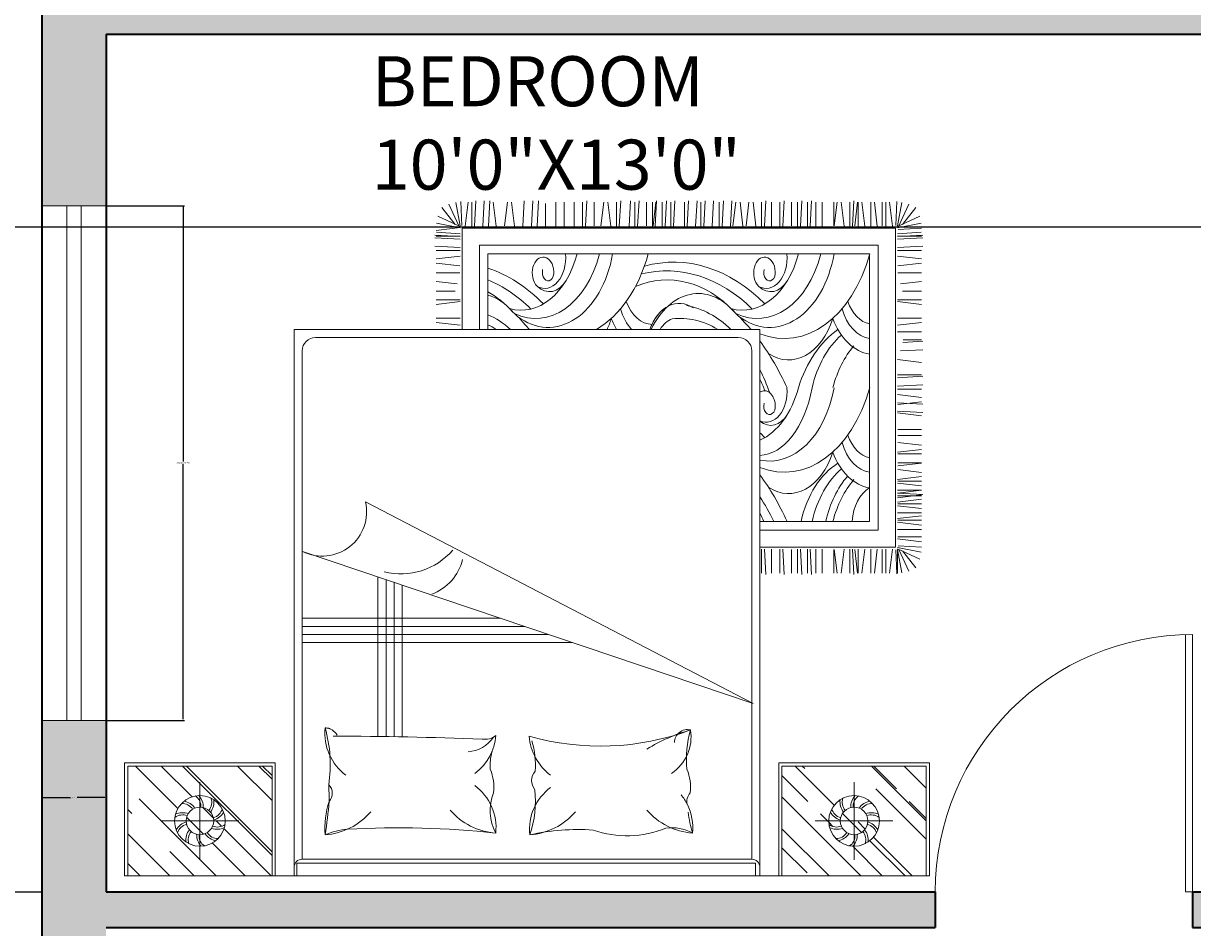
# Model space of a CAD drawing. Units: inches. Extents: x 2540 to 3167, y 3083 to 4007.
# Tile 5 of 15: x 2634 to 2798, y 3416 to 3542. Entities that reach past the tile are written whole.
import ezdxf

# ---------------------------------------------------------------- set-up
doc = ezdxf.new("R2010")
doc.units = ezdxf.units.IN
for name, color, linetype, lineweight in [('A-ANNO-DIMS', 2, 'Continuous', 18), ('A-AREA-IDEN', 7, 'Continuous', 18), ('A-DOOR', 4, 'Continuous', 18), ('A-FLOR-EDGE', 7, 'Continuous', 25), ('A-FURN', 8, 'Continuous', 13), ('A-GLAZ', 4, 'Continuous', 18)]:
    doc.layers.add(name, color=color, linetype=linetype, lineweight=lineweight)
doc.layers.add('A-WALL', color=143, linetype='Continuous', lineweight=35, true_color=0x7aafdf)
doc.layers.add('A-WALL-PATT', color=143, linetype='Continuous', lineweight=13, true_color=0x7aafdf)
doc.styles.get("Standard").update_dxf_attribs({"font": 'arial.ttf'})
doc.dimstyles.get("Standard").update_dxf_attribs({"dimtxt": 0.18, "dimasz": 0.18, "dimexe": 0.18, "dimexo": 0.0625, "dimgap": 0.09, "dimtad": 0, "dimtih": 1, "dimtoh": 1, "dimdec": 4, "dimzin": 0, "dimdsep": 46, "dimtxsty": 'Standard', "dimcen": 0.09, "dimadec": 0, "dimazin": 0, "dimtfac": 1, "dimtdec": 4, "dimtofl": 0, "dimtmove": 0, "dimatfit": 3, "dimfxl": 1, "dimtolj": 1, "dimtzin": 0, "dimarcsym": 0})

# ---------------------------------------------------------------- blocks, each defined once
blk = doc.blocks.new('A$C64B41DC1')
for p, q in [((0, 2.5079), (2.9903, 2.5079)), ((0, 2.0879), (0, 2.5079)), ((0.012, 2.4618), (0.0581, 2.5079)), ((0.012, 2.3515), (0.1684, 2.5079)), ((0.012, 2.0999), (0.012, 2.5079)), ((0.0543, 2.2213), (0.3409, 2.5079)), ((0.1689, 2.4179), (0.2589, 2.5079)), ((0.3265, 2.386), (0.4484, 2.5079)), ((0.3699, 2.3332), (0.5445, 2.5079)), ((0.548, 2.5079), (0.548, 2.0999)), ((0.56, 2.5079), (0.56, 2.0879)), ((0.6301, 2.5079), (0.6301, 0.4779)), ((0.6401, 2.461), (0.6401, 2.5079)), ((0.6401, 2.5079), (2.344, 2.5079)), ((2.344, 2.5079), (2.3601, 2.5079)), ((2.344, 2.5079), (2.344, 2.461)), ((2.3601, 2.5079), (2.3601, 2.4761)), ((2.3601, 0.4779), (2.3601, 2.5079)), ((2.4303, 2.5079), (2.4303, 2.0879)), ((2.4423, 2.5079), (2.4423, 2.0999)), ((2.4423, 2.3333), (2.6169, 2.5079)), ((2.4423, 2.2145), (2.7357, 2.5079)), ((2.4423, 2.404), (2.5354, 2.4971)), ((2.705, 2.398), (2.8149, 2.5079)), ((2.7691, 2.3772), (2.8998, 2.5079)), ((2.7819, 2.3646), (2.9252, 2.5079)), ((2.9783, 2.0999), (2.9783, 2.5079)), ((2.9903, 2.0879), (2.9903, 2.5079)), ((0.2157, 2.0999), (0.548, 2.4322)), ((0.2804, 2.1597), (0.2804, 2.4481)), ((2.344, 2.461), (0.6401, 2.461)), ((0.6601, 2.4461), (1.4951, 2.4461)), ((0.6601, 2.4461), (0.6601, 0.5579)), ((1.4951, 2.4461), (0.6697, 2.4461)), ((2.3301, 2.4461), (1.4951, 2.4461)), ((2.3301, 0.5579), (2.3301, 2.4461)), ((2.7099, 2.1597), (2.7099, 2.4481)), ((0.2299, 2.0999), (0.548, 2.418)), ((0.2311, 2.2906), (0.2937, 2.3532)), ((2.6674, 2.2756), (2.7382, 2.3464)), ((2.7914, 2.1846), (2.9783, 2.3715)), ((0.1362, 2.3039), (0.4246, 2.3039)), ((0.3405, 2.3039), (0.3605, 2.3238)), ((2.8541, 2.3039), (2.5657, 2.3039)), ((2.5849, 2.2779), (2.6158, 2.3088)), ((2.6158, 2.3088), (2.6313, 2.3243)), ((2.7249, 2.3076), (2.7512, 2.3339)), ((2.7746, 2.0999), (2.9783, 2.3036)), ((0.012, 2.261), (0.0275, 2.2765)), ((0.2905, 2.2539), (0.3304, 2.2938)), ((2.9144, 2.2312), (2.9783, 2.2951)), ((0.0404, 2.0999), (0.1982, 2.2578)), ((0.4194, 2.0999), (0.548, 2.2285)), ((2.4423, 2.1353), (2.5382, 2.2312)), ((2.4918, 2.0999), (2.6366, 2.2447)), ((0.1365, 2.0999), (0.251, 2.2144)), ((2.7831, 2.0999), (2.8678, 2.1846)), ((2.8962, 2.0999), (2.9783, 2.182)), ((0.4986, 2.0999), (0.548, 2.1493)), ((0.5127, 2.0999), (0.548, 2.1352)), ((0.56, 2.0879), (0, 2.0879)), ((0.548, 2.0999), (0.012, 2.0999)), ((2.4303, 2.0879), (2.9903, 2.0879)), ((2.4423, 2.0999), (2.9783, 2.0999)), ((2.5172, 2.0999), (2.5269, 2.1096)), ((0.9415, 1.9902), (0.9415, 1.3975)), ((0.9715, 1.9906), (0.9715, 1.4076)), ((1.0015, 1.991), (1.0015, 1.4177)), ((1.0315, 1.9916), (1.0315, 1.4279)), ((2.3349, 1.8678), (0.6613, 1.3029)), ((0.8956, 1.1191), (2.3349, 1.8678)), ((1.6636, 1.6412), (0.6601, 1.6412)), ((1.5748, 1.6112), (0.6601, 1.6112)), ((2.3665, 1.295), (2.3665, 1.3839)), ((2.377, 1.295), (2.3822, 1.3891)), ((2.4032, 1.295), (2.4032, 1.3839)), ((2.4346, 1.295), (2.4346, 1.3839)), ((2.4451, 1.295), (2.4503, 1.3891)), ((2.4774, 1.2957), (2.4774, 1.3837)), ((2.5, 1.295), (2.5, 1.3839)), ((2.5105, 1.295), (2.5157, 1.3891)), ((2.5367, 1.295), (2.5367, 1.3839)), ((2.5471, 1.295), (2.5524, 1.3891)), ((2.5681, 1.295), (2.5681, 1.3839)), ((2.5918, 1.295), (2.5918, 1.3839)), ((2.6346, 1.2957), (2.6346, 1.3837)), ((2.6362, 1.2957), (2.6467, 1.3839)), ((2.6729, 1.295), (2.6624, 1.3839)), ((2.6938, 1.295), (2.6938, 1.3839)), ((2.7043, 1.295), (2.7095, 1.3891)), ((2.7127, 1.2957), (2.7232, 1.3839)), ((2.7253, 1.295), (2.7253, 1.3839)), ((2.7494, 1.295), (2.7389, 1.3839)), ((2.7718, 1.295), (2.7718, 1.3839)), ((2.7959, 1.295), (2.7854, 1.3839)), ((2.8146, 1.2957), (2.8146, 1.3837)), ((2.8146, 1.2957), (2.8146, 1.3837)), ((2.8282, 1.295), (2.8282, 1.3839)), ((2.8282, 1.295), (2.8282, 1.3839)), ((2.8523, 1.295), (2.8418, 1.3839)), ((2.8523, 1.295), (2.8418, 1.3839)), ((2.8653, 1.2966), (2.8688, 1.3861)), ((2.8711, 1.2957), (2.8711, 1.3837)), ((2.8711, 1.2957), (2.8875, 1.3822)), ((2.8765, 1.2958), (2.9132, 1.3758)), ((2.8893, 1.3011), (2.9394, 1.3636)), ((2.8713, 1.2927), (2.954, 1.3315)), ((2.8717, 1.2884), (2.9588, 1.3058)), ((2.3601, 1.2873), (2.8639, 1.2873)), ((2.8639, 1.2873), (2.8639, 0.1018)), ((2.8716, 1.2565), (2.9605, 1.2669)), ((2.8744, 1.2817), (2.9603, 1.2869)), ((2.3601, 1.2233), (2.7999, 1.2233)), ((2.7999, 1.2233), (2.7999, 0.1658)), ((2.8716, 1.2212), (2.9605, 1.2212)), ((2.8723, 1.2489), (2.9603, 1.2489)), ((2.3601, 1.1913), (2.7679, 1.1912)), ((2.7679, 1.1912), (2.7679, 0.1978)), ((2.8716, 1.1947), (2.9605, 1.2052)), ((2.8716, 1.181), (2.9605, 1.1705)), ((2.8723, 1.1872), (2.9603, 1.1872)), ((2.8716, 1.1595), (2.9605, 1.1595)), ((2.8716, 1.133), (2.9605, 1.1435)), ((2.8716, 1.1193), (2.9605, 1.1088)), ((2.8716, 1.1035), (2.9605, 1.093)), ((2.8716, 1.0965), (2.9605, 1.0965)), ((2.8716, 1.086), (2.9657, 1.0913)), ((2.8723, 1.1255), (2.9603, 1.1255)), ((2.8723, 1.0858), (2.9605, 1.0753)), ((2.8716, 1.0756), (2.9605, 1.0756)), ((2.8716, 1.0491), (2.9605, 1.0596)), ((2.8716, 1.0354), (2.9605, 1.0249)), ((2.8723, 1.0416), (2.9603, 1.0416)), ((2.8723, 0.9987), (2.9605, 1.0092)), ((2.8723, 0.985), (2.9605, 0.9745)), ((2.8723, 0.9735), (2.9603, 0.9735)), ((2.8716, 0.9346), (2.9605, 0.9241)), ((2.8723, 0.9408), (2.9603, 0.9408)), ((2.8723, 0.8979), (2.9605, 0.9084)), ((2.8723, 0.8726), (2.9603, 0.8726)), ((2.8723, 0.8505), (2.9603, 0.8505)), ((2.8716, 0.7885), (2.9605, 0.799)), ((2.8716, 0.7818), (2.9657, 0.787)), ((2.8716, 0.7503), (2.9657, 0.7556)), ((2.8723, 0.7571), (2.9605, 0.7466)), ((2.8716, 0.7204), (2.9605, 0.7309)), ((2.8716, 0.6995), (2.9605, 0.6995)), ((2.8716, 0.689), (2.9657, 0.6838)), ((2.8716, 0.6576), (2.9657, 0.6523)), ((2.8716, 0.6471), (2.9605, 0.6471)), ((2.8716, 0.5903), (2.9605, 0.6007)), ((2.882, 0.5582), (2.9657, 0.5536)), ((2.8909, 0.5263), (2.9657, 0.5222)), ((0.6301, 0.4779), (2.3601, 0.4779)), ((0.7101, 0.5079), (2.2801, 0.5079)), ((1.2542, 0.1018), (1.2542, 0.4779)), ((1.3182, 0.1658), (1.3182, 0.4779)), ((1.3502, 0.1978), (1.3502, 0.4779)), ((2.8716, 0.4877), (2.9603, 0.4877)), ((2.8928, 0.5169), (2.9605, 0.5169)), ((1.2465, 0.4625), (1.1576, 0.452)), ((1.2465, 0.4365), (1.1577, 0.4365)), ((2.8716, 0.4625), (2.9605, 0.452)), ((2.8716, 0.4365), (2.9603, 0.4365)), ((1.2465, 0.3746), (1.1576, 0.3851)), ((1.2465, 0.3684), (1.1577, 0.3684)), ((2.8716, 0.3746), (2.9605, 0.3851)), ((2.8716, 0.3684), (2.9603, 0.3684)), ((1.2355, 0.3092), (1.1576, 0.3)), ((1.2285, 0.3357), (1.1577, 0.3357)), ((2.8826, 0.3092), (2.9605, 0.3)), ((2.8896, 0.3357), (2.9603, 0.3357)), ((1.2457, 0.2676), (1.1577, 0.2676)), ((2.8723, 0.2676), (2.9603, 0.2676)), ((1.2457, 0.2423), (1.1576, 0.2319)), ((2.8723, 0.2423), (2.9605, 0.2319)), ((1.2465, 0.1742), (1.1524, 0.169)), ((1.2465, 0.2057), (1.1576, 0.2161)), ((1.2465, 0.1847), (1.1576, 0.1847)), ((2.7679, 0.1978), (1.3502, 0.1978)), ((2.8716, 0.2057), (2.9605, 0.2161)), ((2.8716, 0.1847), (2.9605, 0.1847)), ((2.8716, 0.1742), (2.9657, 0.169)), ((1.2465, 0.1428), (1.1524, 0.1376)), ((1.2465, 0.1334), (1.1524, 0.1281)), ((1.2465, 0.1323), (1.1576, 0.1323)), ((1.2465, 0.1323), (1.1576, 0.1323)), ((2.7999, 0.1658), (1.3182, 0.1658)), ((2.8716, 0.1428), (2.9657, 0.1376)), ((2.8716, 0.1334), (2.9657, 0.1281)), ((2.8716, 0.1323), (2.9605, 0.1323)), ((1.2465, 0.1), (1.1576, 0.1105)), ((1.2465, 0.1229), (1.1588, 0.1168)), ((1.2464, 0.1007), (1.1592, 0.0833)), ((1.2468, 0.0964), (1.1641, 0.0576)), ((1.2288, 0.088), (1.1787, 0.0255)), ((1.2415, 0.0933), (1.2049, 0.0133)), ((1.247, 0.0934), (1.2306, 0.0069)), ((1.2527, 0.0925), (1.2493, 0.003)), ((2.8639, 0.1018), (1.2542, 0.1018)), ((1.2658, 0.0941), (1.2762, 0.0052)), ((1.2899, 0.0941), (1.2899, 0.0052)), ((1.2999, 0.0941), (1.3051, 0)), ((1.3313, 0.0941), (1.3365, 0)), ((1.3523, 0.0941), (1.3575, 0)), ((1.3804, 0.0941), (1.3699, 0.0052)), ((1.4119, 0.0934), (1.4223, 0.0052)), ((1.4485, 0.0941), (1.438, 0.0052)), ((1.48, 0.0941), (1.4852, 0)), ((1.5114, 0.0941), (1.5166, 0)), ((1.5323, 0.0941), (1.5376, 0)), ((1.5638, 0.0941), (1.5638, 0.0105)), ((1.6021, 0.0941), (1.6021, 0.0052)), ((1.6336, 0.0941), (1.6336, 0.0052)), ((1.6702, 0.0941), (1.6702, 0.0052)), ((1.7017, 0.0941), (1.7017, 0.0052)), ((1.7122, 0.0941), (1.7174, 0)), ((1.7445, 0.0934), (1.7445, 0.0054)), ((1.7698, 0.0934), (1.7803, 0.0052)), ((1.8065, 0.0941), (1.796, 0.0052)), ((1.8274, 0.0941), (1.8274, 0.0052)), ((1.8379, 0.0941), (1.8431, 0)), ((1.8746, 0.0941), (1.8798, 0)), ((1.8955, 0.0941), (1.8955, 0.0052)), ((1.906, 0.0941), (1.9113, 0)), ((1.9384, 0.0934), (1.9384, 0.0054)), ((1.9609, 0.0941), (1.9609, 0.0052)), ((1.9636, 0.0934), (1.9741, 0.0052)), ((1.9714, 0.0941), (1.9766, 0)), ((1.9976, 0.0941), (1.9976, 0.0052)), ((2.0081, 0.0941), (2.0133, 0)), ((2.029, 0.0941), (2.029, 0.0052)), ((2.0395, 0.0941), (2.0447, 0)), ((2.0797, 0.0941), (2.0797, 0.0052)), ((2.0902, 0.0941), (2.0954, 0)), ((2.1216, 0.0941), (2.1269, 0)), ((2.1412, 0.0941), (2.1412, 0.0052)), ((2.1517, 0.0941), (2.1569, 0)), ((2.1831, 0.0941), (2.1884, 0)), ((2.2093, 0.0941), (2.2093, 0.0052)), ((2.2198, 0.0941), (2.225, 0)), ((2.2512, 0.0941), (2.2565, 0)), ((2.2603, 0.0934), (2.2707, 0.0052)), ((2.2969, 0.0941), (2.2864, 0.0052)), ((2.3089, 0.0934), (2.3193, 0.0052)), ((2.3455, 0.0941), (2.3351, 0.0052)), ((2.3665, 0.0941), (2.3665, 0.0052)), ((2.377, 0.0941), (2.3822, 0)), ((2.4032, 0.0941), (2.4032, 0.0052)), ((2.4346, 0.0941), (2.4346, 0.0052)), ((2.4451, 0.0941), (2.4503, 0)), ((2.4774, 0.0934), (2.4774, 0.0054)), ((2.5, 0.0941), (2.5, 0.0052)), ((2.5105, 0.0941), (2.5157, 0)), ((2.5367, 0.0941), (2.5367, 0.0052)), ((2.5471, 0.0941), (2.5524, 0)), ((2.5681, 0.0941), (2.5681, 0.0052)), ((2.5918, 0.0941), (2.5918, 0.0052)), ((2.6346, 0.0934), (2.6346, 0.0054)), ((2.6362, 0.0934), (2.6467, 0.0052)), ((2.6729, 0.0941), (2.6624, 0.0052)), ((2.6938, 0.0941), (2.6938, 0.0052)), ((2.7043, 0.0941), (2.7095, 0)), ((2.7127, 0.0934), (2.7232, 0.0052)), ((2.7253, 0.0941), (2.7253, 0.0052)), ((2.7494, 0.0941), (2.7389, 0.0052)), ((2.7718, 0.0941), (2.7718, 0.0052)), ((2.7959, 0.0941), (2.7854, 0.0052)), ((2.8146, 0.0934), (2.8146, 0.0054)), ((2.8282, 0.0941), (2.8282, 0.0052)), ((2.8523, 0.0941), (2.8418, 0.0052)), ((2.8653, 0.0925), (2.8688, 0.003)), ((2.8711, 0.0934), (2.8875, 0.0069)), ((2.8713, 0.0964), (2.954, 0.0576)), ((2.8716, 0.1229), (2.9593, 0.1168)), ((2.8717, 0.1007), (2.9588, 0.0833)), ((2.8744, 0.1074), (2.9603, 0.1022)), ((2.8765, 0.0933), (2.9132, 0.0133)), ((2.8893, 0.088), (2.9394, 0.0255))]:
    blk.add_line(p, q)
at = {"ltscale": 10}
for p, q in [((1.4859, 1.5812), (0.6601, 1.5812)), ((1.397, 1.5512), (0.6601, 1.5512))]:
    blk.add_line(p, q, dxfattribs=at)
for centre, radius in [((0.2804, 2.3039), 0.0942), ((2.7099, 2.3039), 0.0942), ((0.2804, 2.3039), 0.051), ((2.7099, 2.3039), 0.051)]:
    blk.add_circle(centre, radius)
for centre, radius, start, end in [((0.6601, 2.4761), 0.03, 180, 270), ((2.3301, 2.4761), 0.03, 270, 0), ((0.2828, 2.3731), 0.0462, 160.3002, 220.538), ((0.3286, 2.3561), 0.0605, 136.17, 182.4897), ((0.3231, 2.3585), 0.0462, 124.3002, 184.538), ((2.6672, 2.3585), 0.0462, 355.462, 55.6998), ((2.6617, 2.3561), 0.0605, 357.5103, 43.83), ((2.7075, 2.3731), 0.0462, 319.462, 19.6998), ((0.2417, 2.3614), 0.0462, 196.3002, 256.538), ((0.2887, 2.3745), 0.0605, 172.17, 218.4897), ((0.3501, 2.3178), 0.0605, 100.17, 146.4897), ((0.347, 2.323), 0.0462, 88.3002, 148.538), ((1.0526, 2.3302), 0.3085, 175.3048, 198.6942), ((-0.8702, 2.0941), 1.6364, 4.8098, 9.1892), ((0.8579, 2.6278), 0.2948, 247.5179, 264.267), ((0.728, 2.111), 0.245, 40.4189, 85.9871), ((1.0164, 5.7096), 3.3803, 266.8134, 276.1602), ((1.3963, 2.1044), 0.245, 94.0129, 139.5811), ((1.1858, 2.3288), 0.1943, 306.5711, 5.89), ((1.5348, 2.2652), 0.1767, 151.7736, 201.6983), ((1.6986, 2.3355), 0.1943, 174.11, 233.4289), ((1.1481, 2.2311), 0.3783, 353.4947, 19.1867), ((1.6871, 3.192), 0.8561, 257.7438, 273.6284), ((1.4882, 2.111), 0.245, 40.4189, 85.9871), ((1.8674, 1.9709), 0.3878, 68.2026, 108.9817), ((2.1269, 2.1044), 0.245, 94.0129, 139.5811), ((2.0342, 2.4856), 0.1563, 261.5958, 298.9092), ((1.9165, 2.3288), 0.1943, 333.7371, 5.89), ((2.6058, 2.2028), 0.517, 163.6046, 172.3273), ((2.6433, 2.323), 0.0462, 31.462, 91.6998), ((2.6402, 2.3178), 0.0605, 33.5103, 79.83), ((2.7016, 2.3745), 0.0605, 321.5103, 7.83), ((2.7486, 2.3614), 0.0462, 283.462, 343.6998), ((0.2457, 2.3659), 0.0605, 208.17, 254.4897), ((0.3449, 2.2742), 0.0605, 64.17, 110.4897), ((0.3455, 2.2802), 0.0462, 52.3002, 112.538), ((2.6448, 2.2802), 0.0462, 67.462, 127.6998), ((2.6454, 2.2742), 0.0605, 69.5103, 115.83), ((2.7446, 2.3659), 0.0605, 285.5103, 331.83), ((0.2153, 2.3276), 0.0462, 232.3002, 292.538), ((0.2158, 2.3336), 0.0605, 244.17, 290.4897), ((0.2138, 2.2848), 0.0462, 268.3002, 328.538), ((0.2779, 2.2347), 0.0462, 340.3002, 40.538), ((0.272, 2.2333), 0.0605, 352.17, 38.4897), ((0.3191, 2.2464), 0.0462, 16.3002, 76.538), ((0.3151, 2.2419), 0.0605, 28.17, 74.4897), ((2.6752, 2.2419), 0.0605, 105.5103, 151.83), ((2.6712, 2.2464), 0.0462, 103.462, 163.6998), ((2.7182, 2.2333), 0.0605, 141.5103, 187.83), ((2.7123, 2.2347), 0.0462, 139.462, 199.6998), ((2.7765, 2.2848), 0.0462, 211.462, 271.6998), ((2.7744, 2.3336), 0.0605, 249.5103, 295.83), ((2.775, 2.3276), 0.0462, 247.462, 307.6998), ((0.2107, 2.29), 0.0605, 280.17, 326.4897), ((0.2377, 2.2493), 0.0462, 304.3002, 4.538), ((0.2322, 2.2517), 0.0605, 316.17, 2.4897), ((0.7274, 2.2013), 0.0446, 314.4736, 42.1713), ((-1.6008, 2.277), 2.3618, 357.3905, 358.8876), ((1.9165, 2.3288), 0.1943, 320.9404, 333.7371), ((2.1347, 2.2313), 0.0459, 165.3506, 223.2684), ((2.7581, 2.2517), 0.0605, 177.5103, 223.83), ((2.7526, 2.2493), 0.0462, 175.462, 235.6998), ((2.7796, 2.29), 0.0605, 213.5103, 259.83), ((1.204, 2.1778), 0.1681, 337.017, 7.5368), ((1.5671, 2.1546), 0.0547, 142.0833, 220.902), ((1.9346, 2.1778), 0.1681, 337.017, 7.5368), ((0.9385, 1.978), 0.1943, 126.5711, 185.89), ((0.2688, 2.0945), 0.4956, 344.0243, 8.7071), ((1.7059, 1.9714), 0.204, 127.1197, 175.09), ((1.1858, 1.9714), 0.1943, 4.3181, 53.4289), ((1.5415, 2.0969), 0.1834, 175.2233, 196.23), ((1.1965, 2.0983), 0.3299, 343.7954, 3.5554), ((1.9394, 1.991), 0.1651, 351.2621, 55.7572), ((2.4617, 2.0719), 0.3745, 173.8296, 196.4356), ((1.2687, 1.9248), 0.1223, 33.628, 86.4744), ((0.7246, 18.8439), 16.8552, 270.17399, 272.05214), ((1.3401, 1.9404), 0.0603, 49.0991, 101.3702), ((1.7676, 1.0629), 0.9631, 69.6507, 105.9631), ((2.2748, 2.5795), 0.6373, 238.3499, 254.3137), ((2.0911, 2.0123), 0.0478, 179.7727, 283.8018), ((0.7417, 2.0149), 0.057, 273.4709, 328.5412), ((0.728, 2.2025), 0.245, 274.0129, 278.3417), ((1.0747, 1.2871), 0.1871, 14.1863, 69.1212), ((1.0274, 1.1334), 0.2527, 40.629, 104.3712), ((0.7347, 1.1553), 0.1649, 347.3109, 116.4454), ((0.7101, 0.5579), 0.05, 180, 270), ((2.2801, 0.5579), 0.05, 270, 0)]:
    blk.add_arc(centre, radius, start, end)
for centre, major_axis, ratio, start_param, end_param in [((1.9938, 1.6262), (0, -0.7531), 0.68, 0.797284, 0.954936), ((2.0643, 1.466), (0, -0.5322), 0.68, 7.239912, 7.311536), ((1.9052, 1.7397), (0, -0.9842), 0.68, 0.74745, 0.979724), ((2.7455, 1.3081), (0, 0.3614), 0.68, 1.900046, 2.742661), ((2.7868, 1.3081), (0, 0.3614), 0.68, 1.900046, 2.614747), ((2.8372, 1.3081), (0, 0.3614), 0.68, 1.900046, 2.479658), ((2.8607, 1.3211), (0, 0.3614), 0.68, 1.938265, 2.479658), ((2.8057, 1.2079), (0, -0.1524), 0.68, 4.821745, 5.895886), ((2.4665, 0.8216), (0, -0.2664), 0.68, 2.006169, 3.565187), ((2.4513, 0.5069), (0, 0.502), 0.68, 5.095327, 6.553458), ((2.7862, 0.8069), (0, -0.2615), 0.68, 3.244645, 4.205018), ((2.7784, 0.8289), (0, -0.1802), 0.68, 3.227058, 4.318474), ((2.396, 0.6032), (0, 0.3641), 0.68, -1.3172, 0.145284), ((2.3507, 0.5642), (0.0073, 0.3819), 0.56205, -1.21172, -0.009991), ((2.7821, 0.7971), (0, -0.1589), 0.68, 3.272942, 4.229533), ((2.2964, 0.5771), (0, -0.3263), 0.68, 1.938944, 2.850232), ((2.0403, 1.6015), (0, -0.8763), 0.68, 6.849801, 6.887077), ((2.4005, 0.7132), (0, -0.1214), 0.68, 2.284368, 3.652258), ((2.3834, 0.7081), (0, 0.1147), 0.68, 4.593909, 6.585576), ((2.3961, 0.7628), (0, -0.0317), 0.68, 1.462497, 5.046281), ((2.3774, 0.7653), (0, -0.0593), 0.68, 5.841311, 7.755362), ((1.9938, 1.1295), (-0.0678, 0.7439), 0.610498, 3.917146, 4.063997), ((2.0643, 0.9693), (0, -0.5322), 0.68, 7.239912, 7.336618), ((1.9052, 1.243), (0, -0.9842), 0.68, 0.74745, 0.979724), ((2.7455, 0.8114), (-0.0599, 0.3735), 0.695517, 1.775813, 2.548612), ((2.7868, 0.8114), (0, 0.3614), 0.68, 1.900046, 2.614747), ((2.8607, 0.8243), (0, 0.3614), 0.68, 1.938265, 2.479658), ((2.4665, 0.3249), (0, -0.2664), 0.68, 2.006169, 3.565187), ((2.7862, 0.3102), (0, -0.2615), 0.68, 3.244645, 4.205018), ((2.4513, 0.0102), (0, 0.502), 0.68, 5.095327, 6.553458), ((1.242, 0.9693), (0, -0.5322), 0.68, 6.586764, 6.677612), ((1.1714, 1.1295), (-0.1157, 0.7241), 0.59432, 3.291697, 3.50733), ((1.0828, 1.243), (0, -0.9842), 0.68, 0.565948, 0.680366), ((1.5283, 0.0674), (0, -0.3703), 0.68, 1.930561, 3.464283), ((1.5736, 0.1065), (0, 0.3641), 0.68, -1.3172, 0.476403), ((1.6289, 0.0102), (0, 0.502), 0.68, 6.655152, 6.661293), ((1.6289, 0.0102), (0, 0.502), 0.68, 5.095327, 5.911219), ((1.6442, 0.3249), (0, -0.2664), 0.68, 2.006169, 2.182797), ((1.9638, 0.3102), (0, -0.2615), 0.68, 4.015924, 4.205018), ((1.956, 0.3322), (0, -0.1802), 0.68, 3.770744, 4.318474), ((2.0606, 0.5616), (0, -0.1803), 0.68, 5.194792, 5.929328), ((2.0606, 0.5616), (0, -0.1803), 0.68, 5.194792, 6.723255), ((2.1315, 0.6603), (0, -0.3155), 0.68, 5.328638, 6.949396), ((2.0549, 0.5656), (0, -0.1303), 0.68, 5.450951, 6.054641), ((2.0643, 0.9693), (0, -0.5322), 0.68, 6.20013, 6.677612), ((1.9938, 1.1295), (-0.0678, 0.7439), 0.610498, 3.199135, 3.592282), ((1.9052, 1.243), (0, -0.9842), 0.68, 0.565948, 0.680366), ((2.3507, 0.0674), (0, -0.3703), 0.68, 1.930561, 3.464283), ((2.396, 0.1065), (0, 0.3641), 0.68, -1.3172, 0.476403), ((2.4513, 0.0102), (0, 0.502), 0.68, 6.655152, 6.661293), ((2.7784, 0.3322), (0, -0.1802), 0.68, 3.227058, 4.318474), ((1.9597, 0.3004), (0, -0.1589), 0.68, 3.14258, 4.229533), ((2.7821, 0.3004), (0, -0.1589), 0.68, 3.272942, 4.229533), ((1.1933, 0.9181), (0, -0.624), 0.68, 0.378672, 0.625379), ((1.3091, 0.6603), (0, -0.3155), 0.68, 6.475719, 6.949396), ((1.1911, 1.1066), (0, 0.8458), 0.68, 3.421828, 3.728616), ((1.474, 0.0804), (0, -0.3263), 0.68, 1.938944, 3.339184), ((2.0157, 0.9181), (0, -0.624), 0.68, -0.280078, 0.625379), ((2.0135, 1.1066), (0, 0.8458), 0.68, 2.978727, 3.728616), ((2.2964, 0.0804), (0, -0.3263), 0.68, 1.938944, 3.339184), ((1.2179, 1.1047), (0, -0.8763), 0.68, 6.507006, 6.887077), ((1.5781, 0.2165), (0, -0.1214), 0.68, 2.284368, 3.726131), ((2.0403, 1.1047), (0, -0.8763), 0.68, 6.099302, 6.887077), ((2.4005, 0.2165), (0, -0.1214), 0.68, 2.284368, 3.726131), ((1.555, 0.2685), (0, -0.0593), 0.68, 3.732151, 7.755362), ((1.561, 0.2114), (0, 0.1147), 0.68, 4.593909, 6.647252), ((2.3774, 0.2685), (0, -0.0593), 0.68, 3.732151, 7.755362), ((2.3834, 0.2114), (0, 0.1147), 0.68, 4.593909, 6.647252), ((1.5737, 0.2661), (0, -0.0317), 0.68, 1.462497, 5.046281), ((2.3961, 0.2661), (0, -0.0317), 0.68, 1.462497, 5.046281)]:
    blk.add_ellipse(centre, major_axis=major_axis, ratio=ratio, start_param=start_param, end_param=end_param)
blk = doc.blocks.new('DOOR-SWING-36IN')
for p, q in [((36, 0), (0, 0)), ((36, 1), (0.01, 1)), ((36, 1), (36, 0))]:
    blk.add_line(p, q)
blk.add_arc((36, 0), 36, 90, 180)
blk = doc.blocks.new('WIN-72IN')
for p, q in [((9, 72), (0, 72)), ((3.5, 0), (3.5, 72)), ((5.5, 0), (5.5, 72)), ((9, 0), (0, 0))]:
    blk.add_line(p, q)
blk = doc.blocks.new('*D27')
at = {"layer": 'A-ANNO-DIMS', "color": 0, "lineweight": -2, "transparency": 16777216}
for p, q in [((2645.57, 3516.71), (2656.49, 3516.71)), ((2656.31, 3516.53), (2656.31, 3480.9)), ((2656.31, 3444.89), (2656.31, 3480.53)), ((2645.57, 3444.71), (2656.49, 3444.71))]:
    blk.add_line(p, q, dxfattribs=at)
at = {"layer": 'A-ANNO-DIMS', "color": 0, "transparency": 16777216}
for points in [[(2656.28, 3516.53), (2656.34, 3516.53), (2656.31, 3516.71)], [(2656.28, 3444.89), (2656.34, 3444.89), (2656.31, 3444.71)]]:
    blk.add_solid(points, dxfattribs=at)
at = {"layer": 'Defpoints', "color": 0, "transparency": 16777216}
for p in [(2645.51, 3516.71), (2656.31, 3516.71), (2645.51, 3444.71)]:
    blk.add_point(p, dxfattribs=at)
at = {"layer": 'A-ANNO-DIMS', "color": 0, "transparency": 16777216, "insert": (2656.31, 3480.71), "char_height": 0.18, "attachment_point": 5}
blk.add_mtext('\\A1;WINDOW 72 TYP.', dxfattribs=at)
blk = doc.blocks.new('*D28')
at = {"layer": 'A-ANNO-DIMS', "color": 0, "lineweight": -2, "transparency": 16777216}
for p, q in [((2636.51, 3444.65), (2636.51, 3433.73)), ((2645.51, 3444.65), (2645.51, 3433.73)), ((2636.69, 3433.91), (2640.55, 3433.91)), ((2645.33, 3433.91), (2641.47, 3433.91))]:
    blk.add_line(p, q, dxfattribs=at)
at = {"layer": 'A-ANNO-DIMS', "color": 0, "transparency": 16777216}
for points in [[(2636.69, 3433.94), (2636.69, 3433.88), (2636.51, 3433.91)], [(2645.33, 3433.94), (2645.33, 3433.88), (2645.51, 3433.91)]]:
    blk.add_solid(points, dxfattribs=at)
at = {"layer": 'Defpoints', "color": 0, "transparency": 16777216}
for p in [(2636.51, 3444.71), (2645.51, 3444.71), (2645.51, 3433.91)]:
    blk.add_point(p, dxfattribs=at)
at = {"layer": 'A-ANNO-DIMS', "color": 0, "transparency": 16777216, "insert": (2641.01, 3433.91), "char_height": 0.18, "attachment_point": 5}
blk.add_mtext('\\A1;9 TYP.', dxfattribs=at)
blk = doc.blocks.new('*D44')
at = {"layer": 'A-ANNO-DIMS', "color": 0, "lineweight": -2, "transparency": 16777216}
for p, q in [((2771.45, 3964.71), (2540.23, 3964.71)), ((2540.41, 3964.53), (2540.41, 3545.4)), ((2540.41, 3125.89), (2540.41, 3545.03)), ((2810.45, 3125.71), (2540.23, 3125.71))]:
    blk.add_line(p, q, dxfattribs=at)
at = {"layer": 'A-ANNO-DIMS', "color": 0, "transparency": 16777216}
for points in [[(2540.38, 3964.53), (2540.44, 3964.53), (2540.41, 3964.71)], [(2540.38, 3125.89), (2540.44, 3125.89), (2540.41, 3125.71)]]:
    blk.add_solid(points, dxfattribs=at)
at = {"layer": 'Defpoints', "color": 0, "transparency": 16777216}
for p in [(2540.41, 3964.71), (2771.51, 3964.71), (2810.51, 3125.71)]:
    blk.add_point(p, dxfattribs=at)
at = {"layer": 'A-ANNO-DIMS', "color": 0, "transparency": 16777216, "insert": (2540.41, 3545.21), "char_height": 0.18, "attachment_point": 5}
blk.add_mtext('\\A1;839', dxfattribs=at)
blk = doc.blocks.new('*D57')
at = {"layer": 'A-ANNO-DIMS', "color": 0, "lineweight": -2, "transparency": 16777216}
for p, q in [((2810.45, 3564.71), (2540.23, 3564.71)), ((2540.41, 3564.53), (2540.41, 3539.4)), ((2540.41, 3513.89), (2540.41, 3539.03)), ((2810.45, 3513.71), (2540.23, 3513.71))]:
    blk.add_line(p, q, dxfattribs=at)
at = {"layer": 'A-ANNO-DIMS', "color": 0, "transparency": 16777216}
for points in [[(2540.38, 3564.53), (2540.44, 3564.53), (2540.41, 3564.71)], [(2540.38, 3513.89), (2540.44, 3513.89), (2540.41, 3513.71)]]:
    blk.add_solid(points, dxfattribs=at)
at = {"layer": 'Defpoints', "color": 0, "transparency": 16777216}
for p in [(2810.51, 3564.71), (2540.41, 3513.71), (2810.51, 3513.71)]:
    blk.add_point(p, dxfattribs=at)
at = {"layer": 'A-ANNO-DIMS', "color": 0, "transparency": 16777216, "insert": (2540.41, 3539.21), "char_height": 0.18, "attachment_point": 5}
blk.add_mtext('\\A1;51', dxfattribs=at)

msp = doc.modelspace()

# ---------------------------------------------------------------- hatches: boundary and pattern name
at = {"layer": 'A-WALL-PATT'}
h = msp.add_hatch(color=256, dxfattribs=at)
h.dxf.hatch_style = 1
h.paths.add_polyline_path([(2805.51, 3803.71), (2800.51, 3803.71), (2800.51, 3799.71), (2621.51, 3799.71), (2621.51, 3823.71), (2612.51, 3823.71), (2612.51, 3794.71), (2636.51, 3794.71), (2636.51, 3782.71), (2645.51, 3782.71), (2645.51, 3794.71), (2805.51, 3794.71)])
h.paths.add_polyline_path([(2810.51, 3564.71), (2868.51, 3564.71), (2868.51, 3627.71), (2872.51, 3627.71), (2872.51, 3636.71), (2864.51, 3636.71), (2864.51, 3674.71), (2797.51, 3674.71), (2797.51, 3669.71), (2801.51, 3669.71), (2801.51, 3628.63), (2806.51, 3628.63), (2806.51, 3669.71), (2859.51, 3669.71), (2859.51, 3573.71), (2806.51, 3573.71), (2806.51, 3598.63), (2801.51, 3598.63), (2801.51, 3549.71), (2645.51, 3549.71), (2645.51, 3573.71), (2636.51, 3573.71), (2636.51, 3516.71), (2645.51, 3516.71), (2645.51, 3540.71), (2801.51, 3540.71), (2801.51, 3504.71), (2801.51, 3500.71), (2806.51, 3500.71), (2806.51, 3504.71), (2859.51, 3504.71), (2859.51, 3420.71), (2806.51, 3420.71), (2806.51, 3470.71), (2801.51, 3470.71), (2801.51, 3420.71), (2797.51, 3420.71), (2797.51, 3415.71), (2864.51, 3415.71), (2864.51, 3453.71), (2868.51, 3453.71), (2868.51, 3513.71), (2810.51, 3513.71)])
h.paths.add_polyline_path([(2645.51, 3415.71), (2761.51, 3415.71), (2761.51, 3420.71), (2645.51, 3420.71), (2645.51, 3444.71), (2636.51, 3444.71), (2636.51, 3403.71), (2645.51, 3403.71)])
h.paths.add_polyline_path([(2645.51, 3307.71), (2636.51, 3307.71), (2636.51, 3295.71), (2612.51, 3295.71), (2612.51, 3149.71), (2645.51, 3149.71), (2645.51, 3158.71), (2621.51, 3158.71), (2621.51, 3290.71), (2801.51, 3290.71), (2801.51, 3286.71), (2806.51, 3286.71), (2806.51, 3295.71), (2645.51, 3295.71)])
h.paths.add_polyline_path([(2762.01, 3158.71), (2746.51, 3158.71), (2746.51, 3240.71), (2750.51, 3240.71), (2750.51, 3245.71), (2741.51, 3245.71), (2741.51, 3158.71), (2717.51, 3158.71), (2717.51, 3149.71), (2762.01, 3149.71)], flags=17)
h.paths.add_polyline_path([(2810.51, 3173.71), (2822.51, 3173.71), (2822.51, 3182.71), (2806.51, 3182.71), (2806.51, 3250.71), (2801.51, 3250.71), (2801.51, 3245.71), (2780.51, 3245.71), (2780.51, 3240.71), (2801.51, 3240.71), (2801.51, 3158.71), (2786.01, 3158.71), (2786.01, 3149.71), (2810.51, 3149.71)])
h.paths.add_polyline_path([(2931.51, 3290.71), (2935.51, 3290.71), (2935.51, 3295.71), (2926.51, 3295.71), (2926.51, 3182.71), (2910.51, 3182.71), (2910.51, 3173.71), (2922.51, 3173.71), (2922.51, 3149.71), (2987.51, 3149.71), (2987.51, 3158.71), (2931.51, 3158.71)])
h.paths.add_polyline_path([(3124.51, 3295.71), (3086.51, 3295.71), (3018.51, 3295.71), (3018.51, 3290.71), (3115.51, 3290.71), (3115.51, 3158.71), (3059.51, 3158.71), (3059.51, 3149.71), (3124.51, 3149.71)])
h.paths.add_polyline_path([(2988.51, 3295.71), (2984.51, 3295.71), (2984.51, 3349.71), (3086.51, 3349.71), (3086.51, 3320.71), (3124.51, 3320.71), (3124.51, 3354.71), (3071.51, 3354.71), (3071.51, 3358.71), (3062.51, 3358.71), (3062.51, 3354.71), (2979.51, 3354.71), (2979.51, 3295.71), (2971.51, 3295.71), (2971.51, 3290.71), (2988.51, 3290.71)])
h.paths.add_polyline_path([(3095.51, 3325.71), (3095.51, 3349.71), (3119.51, 3349.71), (3119.51, 3325.71)], flags=16)
h.paths.add_polyline_path([(3124.51, 3462.71), (3071.51, 3462.71), (3071.51, 3627.71), (3124.51, 3627.71), (3124.51, 3693.71), (3095.51, 3693.71), (3095.51, 3702.71), (3086.51, 3702.71), (3086.51, 3684.71), (3086.51, 3636.71), (2930.51, 3636.71), (2930.51, 3768.71), (2934.51, 3768.71), (2934.51, 3773.71), (2930.51, 3773.71), (2925.51, 3773.71), (2925.51, 3730.71), (2864.51, 3730.71), (2864.51, 3760.71), (2859.51, 3760.71), (2859.51, 3725.71), (2925.51, 3725.71), (2925.51, 3636.71), (2908.51, 3636.71), (2908.51, 3627.71), (3062.51, 3627.71), (3062.51, 3543.71), (2930.51, 3543.71), (2930.51, 3534.71), (2993.51, 3534.71), (2993.51, 3516.71), (3002.51, 3516.71), (3002.51, 3534.71), (3062.51, 3534.71), (3062.51, 3462.71), (3002.51, 3462.71), (3002.51, 3480.71), (2993.51, 3480.71), (2993.51, 3462.71), (2916.51, 3462.71), (2916.51, 3453.71), (2926.51, 3453.71), (2926.51, 3361.71), (2859.51, 3361.71), (2859.51, 3338.71), (2864.51, 3338.71), (2864.51, 3356.71), (2926.51, 3356.71), (2926.51, 3338.71), (2931.51, 3338.71), (2931.51, 3453.71), (3062.51, 3453.71), (3062.51, 3448.21), (3071.51, 3448.21), (3071.51, 3453.71), (3124.51, 3453.71)])

# ---------------------------------------------------------------- linework, layer by layer
at = {"layer": 'A-FLOR-EDGE'}
msp.add_line((2588.51, 3420.71), (2636.51, 3420.71), dxfattribs=at)
at = {"layer": 'A-WALL'}
for p, q in [((2636.51, 3686.71), (2636.51, 3403.71)), ((2645.51, 3540.71), (2801.51, 3540.71)), ((2645.51, 3540.71), (2645.51, 3420.71)), ((2645.51, 3420.71), (2761.51, 3420.71)), ((2761.51, 3420.71), (2761.51, 3415.71)), ((2797.51, 3420.71), (2797.51, 3415.71)), ((2797.51, 3420.71), (2801.51, 3420.71)), ((2645.51, 3415.71), (2761.51, 3415.71)), ((2797.51, 3415.71), (2864.51, 3415.71))]:
    msp.add_line(p, q, dxfattribs=at)

# ---------------------------------------------------------------- block references
at = {"layer": 'A-DOOR', "extrusion": (0, 0, -1), "zscale": -1, "rotation": 270.0000000000015}
msp.add_blockref('DOOR-SWING-36IN', (-2797.51, 3456.71), dxfattribs=at)
at = {"layer": 'A-FURN', "xscale": -37.66426153275995, "yscale": 37.66426153275995, "zscale": 37.66426153275995, "rotation": 180}
msp.add_blockref('A$C64B41DC1', (2648.08, 3517.41), dxfattribs=at)
at = {"layer": 'A-GLAZ'}
msp.add_blockref('WIN-72IN', (2636.51, 3444.71), dxfattribs=at)

# ---------------------------------------------------------------- texts
at = {"layer": 'A-AREA-IDEN', "insert": (2682.68, 3537.62), "char_height": 7, "attachment_point": 1}
msp.add_mtext_dynamic_manual_height_columns('BEDROOM\\P10\'0"X13\'0"', width=74.1323, gutter_width=12.5, heights=[0], dxfattribs=at)

# ---------------------------------------------------------------- dimensions: what is measured, and where the dimension line sits
at = {"layer": 'A-ANNO-DIMS'}
for base, p1, p2, picture, middle in [((2540.41, 3964.71), (2810.51, 3125.71), (2771.51, 3964.71), '*D44', (2540.41, 3545.21)), ((2540.41, 3513.71), (2810.51, 3564.71), (2810.51, 3513.71), '*D57', (2540.41, 3539.21))]:
    dim = msp.add_linear_dim(base=base, p1=p1, p2=p2, angle=90, dimstyle='Standard', override={"dimdec": 0, "dimlfac": 1, "dimrnd": 0, "dimzin": 0, "dimdsep": 46, "dimlunit": 2}, dxfattribs=at)
    dim.commit()
    dim.dimension.update_dxf_attribs({"geometry": picture, "text_midpoint": middle})
dim = msp.add_linear_dim(base=(2656.31, 3516.71), p1=(2645.51, 3444.71), p2=(2645.51, 3516.71), angle=90, text='WINDOW <> TYP.', dimstyle='Standard', override={"dimdec": 0, "dimlfac": 1, "dimrnd": 0, "dimzin": 0, "dimdsep": 46, "dimlunit": 2}, dxfattribs=at)
dim.commit()
dim.dimension.update_dxf_attribs({"geometry": '*D27', "text_midpoint": (2656.31, 3480.71)})
dim = msp.add_linear_dim(base=(2645.51, 3433.91), p1=(2636.51, 3444.71), p2=(2645.51, 3444.71), text='<> TYP.', dimstyle='Standard', override={"dimdec": 0, "dimlfac": 1, "dimrnd": 0, "dimzin": 0, "dimdsep": 46, "dimlunit": 2}, dxfattribs=at)
dim.commit()
dim.dimension.update_dxf_attribs({"geometry": '*D28', "text_midpoint": (2641.01, 3433.91)})

doc.saveas('drawing.dxf')
